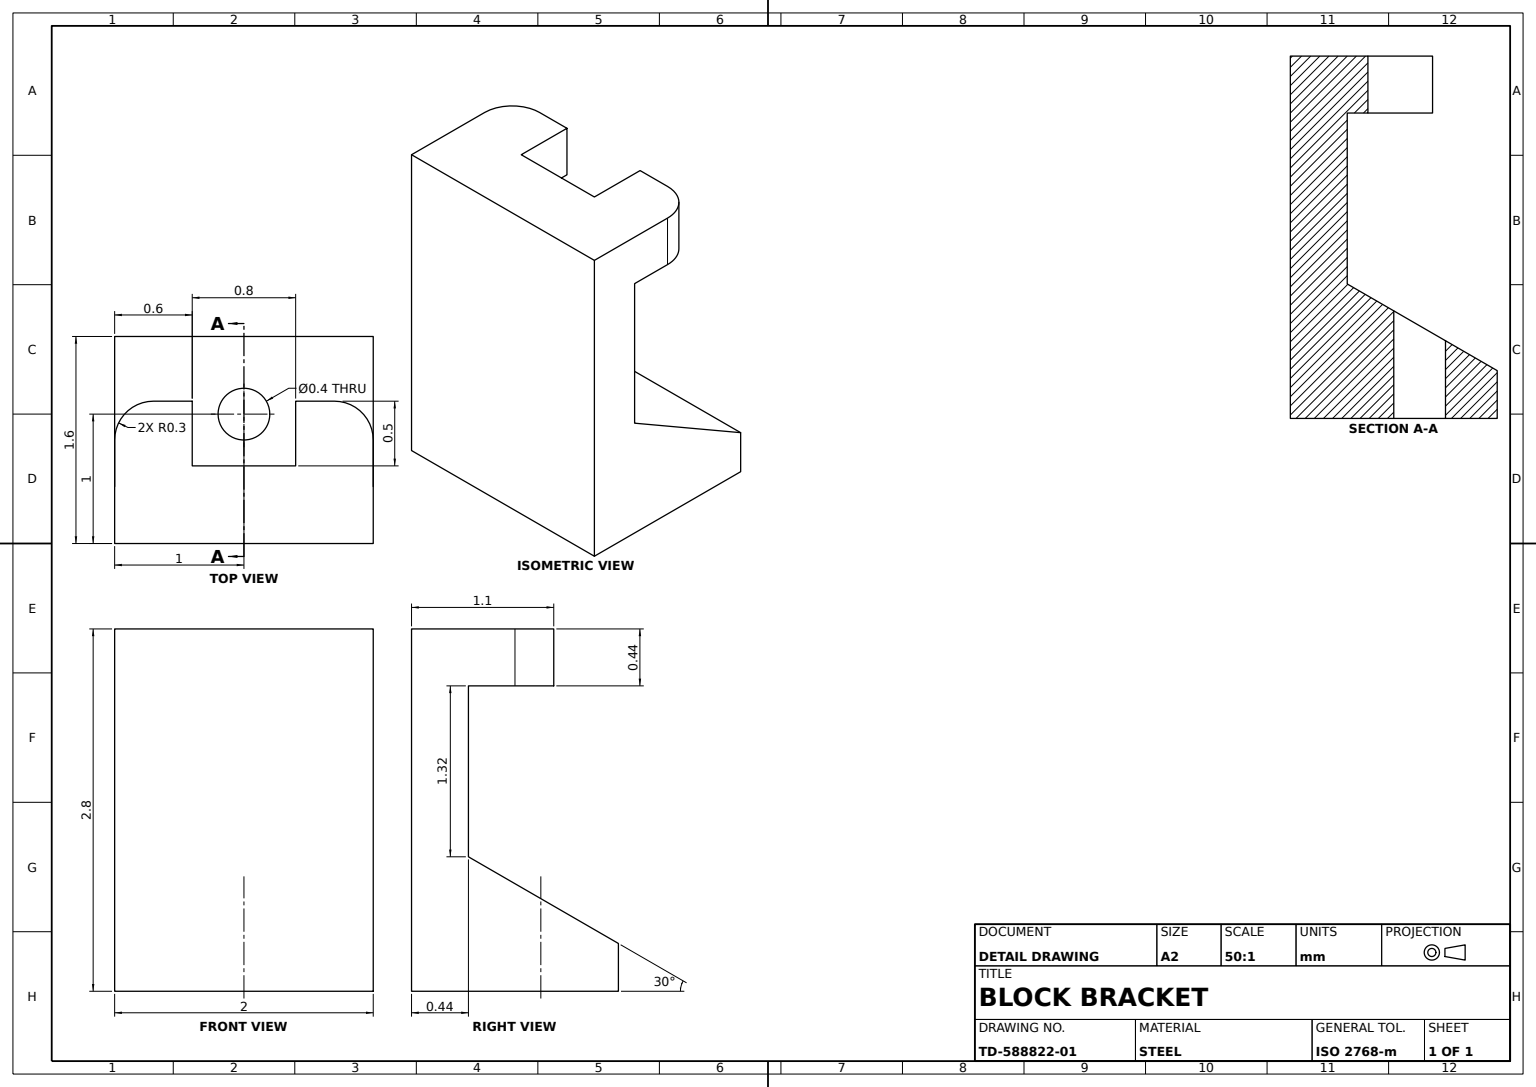
SolidWorks part; units mm, degrees
material "Plain Carbon Steel"
ref_plane "Front Plane" through (0, 0, 0) normal (0, 0, 1) x (1, 0, 0)
ref_plane "Top Plane" through (0, 0, 0) normal (0, 1, 0) x (1, 0, 0)
ref_plane "Right Plane" through (0, 0, 0) normal (1, 0, 0) x (0, 0, -1)
sketch "C-Profile Sketch" plane through (0, 0, 0) normal (0, 0, 1) x (1, 0, 0)
  line L0 (0, 0) -> (1.6, 0)
  line L1 (1.6, 0) -> (1.6, 2.8)
  line L2 (1.6, 2.8) -> (0.5, 2.8)
  line L3 (0.5, 2.8) -> (0.5, 2.36)
  line L6 (0, 0) -> (0, 0.3694)
  line L7 (1.16, 2.36) -> (1.16, 1.0391)
  line L8 (1.16, 2.36) -> (0.5, 2.36)
  line L9 (0, 0.3694) -> (1.16, 1.0391)
  dimension "D1" = 30
  dimension "D2" = 2.8
  dimension "D3" = 1.6
  dimension "D4" = 0.44
  dimension "D5" = 1.1
  dimension "D6" = 0.44
  dimension "D7" = 1.0391
extrude "C-Bracket Body" add sketch "C-Profile Sketch" against normal blind 2
sketch "Recess Cut A Sketch" plane through (0, 2.8, 0) normal (0, 1, 0) x (1, 0, 0)
  line L0 (0.5, 2) -> (0.8, 2)
  line L1 (1.6, 2) -> (0.5, 2) construction
  line L2 (0.5, 0) -> (0.8, 0)
  line L3 (0.5, 2) -> (0.5, 1.7)
  line L4 (1.6, 0) -> (0.5, 0) construction
  line L6 (0.5, 0) -> (0.5, 0.3)
  arc A0 (0.8, 2) -> (0.5, 1.7) centre (0.8, 1.7) ccw
  arc A1 (0.5, 0.3) -> (0.8, 0) centre (0.8, 0.3) ccw
  dimension "D1" = 0.3
extrude "Recess Cut A 0.44 Deep" cut sketch "Recess Cut A Sketch" against normal blind 0.44
sketch "Recess Cut B Sketch" plane through (0, 2.8, 0) normal (0, 1, 0) x (1, 0, 0)
  line L2 (1, 1) -> (1, 1.4)
  line L3 (1, 1.4) -> (0.5, 1.4)
  line L4 (0.5, 1.7) -> (0.5, 0.3) construction
  line L5 (0.5, 1.4) -> (0.5, 0.6)
  line L6 (0.5, 0.6) -> (1, 0.6)
  line L7 (1, 0.6) -> (1, 1)
  dimension "D1" = 0.5
  dimension "D2" = 0.6
  dimension "D3" = 1
extrude "Recess Cut B 0.44 Deep" cut sketch "Recess Cut B Sketch" against normal blind 0.44
sketch "Hole Sketch" plane through (0, 0, 0) normal (0, -1, 0) x (1, 0, 0)
  line L0 (0, -2) -> (0, 0) construction
  line L1 (0, 0) -> (1.6, 0) construction
  circle A0 centre (0.6, -1) radius 0.2
  dimension "D1" = 0.4
  dimension "D2" = 0.4
  dimension "D3" = 0.6
  dimension "D4" = 1
extrude "Hole Ø0.4 x 1 Deep" cut sketch "Hole Sketch" against normal blind 1
